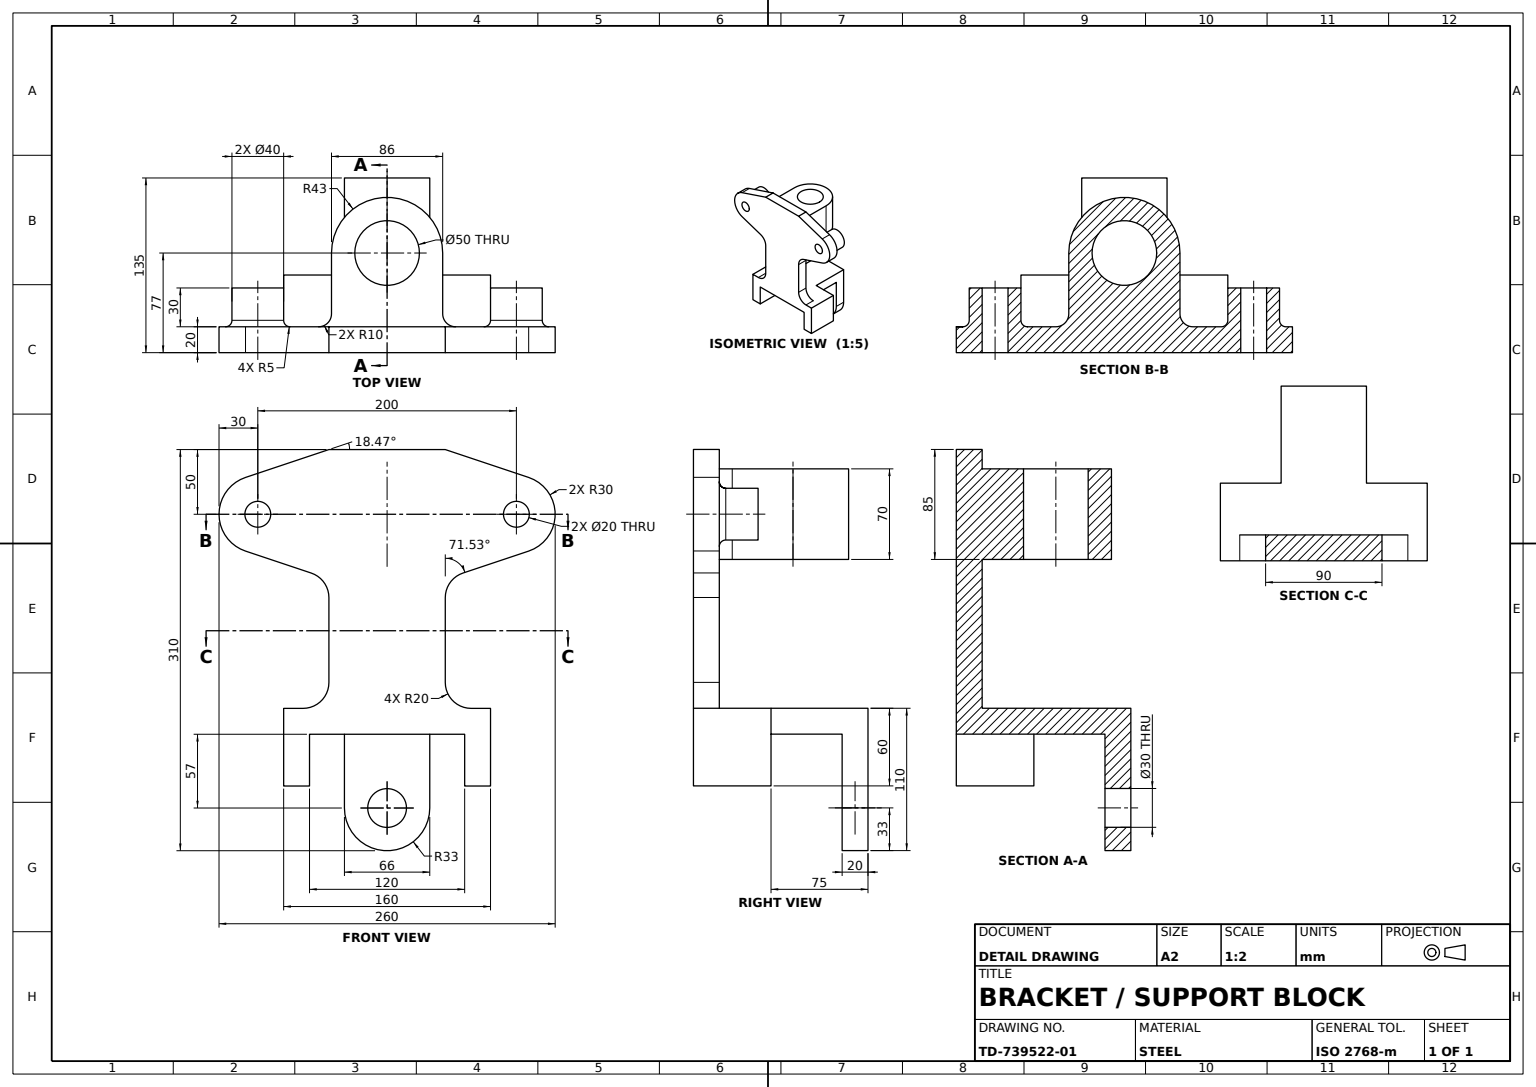
from build123d import *

# Parameters (mm, degrees)
BASE_BODY_DEPTH          = 20
HUB_BOSS_SKETCH_R        = 20
HUB_BOSS_DEPTH           = 30
HUB_BORE_SKETCH_R        = 10
HUB_BORE_20_DEPTH        = 205.694894905
FOOT_BLOCK_SKETCH_R      = 25
FOOT_BLOCK_DEPTH         = 35
HINGE_PLATE_DEPTH        = 20
PLATE_STIFFENER_SKETCH_R = 15
PLATE_STIFFENER_DEPTH    = 20
PIN_BOSS_SKETCH_W        = 60
PIN_BOSS_SKETCH_H        = 60
PIN_BOSS_DEPTH           = 20
HUB_FILLET_R5_R          = 5
FOOT_BLOCK_FILLET_R10_R  = 10
HINGE_PLATE_FILLET_R20_R = 20


with BuildPart() as part:
    # Base Profile Sketch → Base Body (new body)
    with BuildSketch(Plane(origin=(0, 0, 0), x_dir=(0, 0, -1), z_dir=(1, 0, 0))):
        with BuildLine():
            Line((45, 50), (-45, 50))
            Line((-45, 50), (-109.504258609, 28.45468447))
            ThreePointArc((-109.504258609, 28.45468447), (-130, 0), (-109.504258609, -28.45468447))
            Line((-109.504258609, -28.45468447), (-58.663827594, -45.436092388))
            ThreePointArc((-58.663827594, -45.436092388), (-48.771576661, -52.716644423), (-45, -64.405882035))
            Line((-45, -64.405882035), (-45, -150))
            Line((-45, -150), (45, -150))
            Line((45, -150), (45, -64.405882035))
            ThreePointArc((45, -64.405882035), (48.771576661, -52.716644423), (58.663827594, -45.436092388))
            Line((58.663827594, -45.436092388), (109.504258609, -28.45468447))
            ThreePointArc((109.504258609, -28.45468447), (130, 0), (109.504258609, 28.45468447))
            Line((109.504258609, 28.45468447), (45, 50))
        make_face()
    extrude(amount=BASE_BODY_DEPTH)

    # Hub Boss Sketch → Hub Boss (add)
    with BuildSketch(Plane.ZY):
        with Locations(Location((-100, 0, 0), (0, 0, 180))):
            Circle(HUB_BOSS_SKETCH_R)
        with Locations(Location((100, 0, 0), (0, 0, 180))):
            Circle(HUB_BOSS_SKETCH_R)
    extrude(amount=HUB_BOSS_DEPTH)

    # Hub Bore Sketch → Hub Bore Ø20 (cut, through all)
    with BuildSketch(Plane.ZY.offset(30)):
        with Locations((-100, 0)):
            Circle(HUB_BORE_SKETCH_R)
        with Locations((100, 0)):
            Circle(HUB_BORE_SKETCH_R)
    extrude(amount=-HUB_BORE_20_DEPTH, mode=Mode.SUBTRACT)

    # Foot Block Sketch → Foot Block (add, symmetric)
    with BuildSketch(Plane(origin=(0, 0, 0), x_dir=(1, 0, 0), z_dir=(0, 1, 0))):
        with BuildLine():
            Line((-57, 43), (0, 43))
            Line((0, 43), (0, -43))
            Line((0, -43), (-57, -43))
            ThreePointArc((-57, -43), (-100, 0), (-57, 43))
        make_face()
        with Locations(Location((-57, 0, 0), (0, 0, 270))):
            Circle(FOOT_BLOCK_SKETCH_R, mode=Mode.SUBTRACT)
    extrude(amount=FOOT_BLOCK_DEPTH, both=True)

    # Hinge Plate Sketch → Hinge Plate (add)
    with BuildSketch(Plane.XZ.offset(150)):
        Polygon((20, 0), (20, 80), (-40, 80), (-40, 33), (-115, 33), (-115, -33), (-40, -33), (-40, -80), (20, -80), align=None)
    extrude(amount=HINGE_PLATE_DEPTH)

    # Plate Stiffener Sketch → Plate Stiffener (add)
    with BuildSketch(Plane.ZY.offset(115)):
        with BuildLine():
            Line((-33, -150), (33, -150))
            Line((33, -150), (33, -227))
            ThreePointArc((33, -227), (0, -260), (-33, -227))
            Line((-33, -227), (-33, -150))
        make_face()
        with Locations((0, -227)):
            Circle(PLATE_STIFFENER_SKETCH_R, mode=Mode.SUBTRACT)
    extrude(amount=-PLATE_STIFFENER_DEPTH)

    # Pin Boss Sketch → Pin Boss (add)
    with BuildSketch(Plane.XY.offset(80)):
        with Locations((-10, -180)):
            Rectangle(PIN_BOSS_SKETCH_W, PIN_BOSS_SKETCH_H)
    pin_boss = extrude(amount=-PIN_BOSS_DEPTH)

    # Pin Boss Mirror: Pin Boss across plane
    add(pin_boss.mirror(Plane.XY))

    # Hub Fillet R5
    hub_fillet_r5_edges = [part.edges().sort_by_distance(p)[0] for p in [
        (0, 0, -80),
        (0, 0, 120),
    ]]
    fillet(hub_fillet_r5_edges, radius=HUB_FILLET_R5_R)

    # Foot Block Fillet R10
    foot_block_fillet_r10_edges = [part.edges().sort_by_distance(p)[0] for p in [
        (0, 0, 43),
        (0, 0, -43),
    ]]
    fillet(foot_block_fillet_r10_edges, radius=FOOT_BLOCK_FILLET_R10_R)

    # Hinge Plate Fillet R20
    hinge_plate_fillet_r20_edges = [part.edges().sort_by_distance(p)[0] for p in [
        (10, -150, -45),
        (10, -150, 45),
    ]]
    fillet(hinge_plate_fillet_r20_edges, radius=HINGE_PLATE_FILLET_R20_R)


solid = part.part
